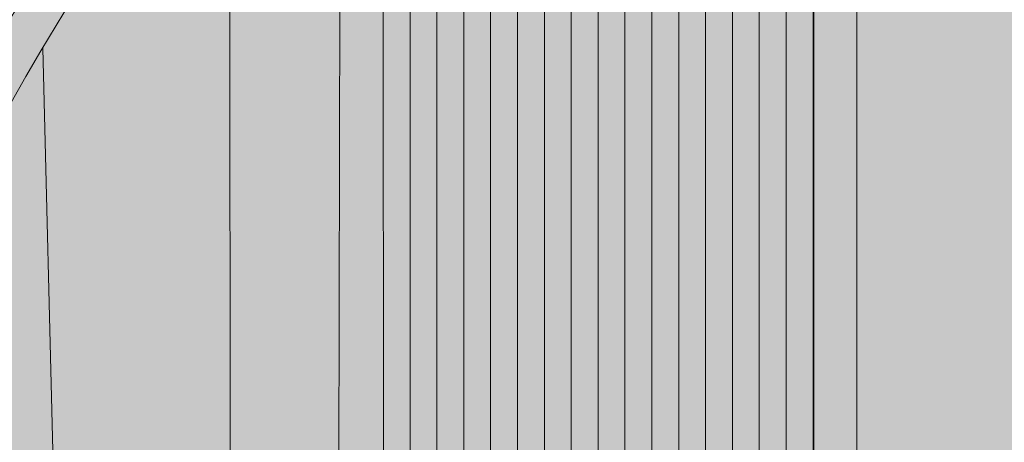
# Model space of a CAD drawing. Units: millimetres. Extents: x 11032 to 26788, y 3406 to 24505.
# Tile 9 of 78: x 15421 to 16566, y 8278 to 8770. Entities that reach past the tile are written whole.
import ezdxf

# ---------------------------------------------------------------- set-up
doc = ezdxf.new("R2010")
doc.units = ezdxf.units.MM
doc.header["$MEASUREMENT"] = 0
for name, color, linetype, lineweight in [('A-ANNO-DIMS', 2, 'Continuous', 18), ('A-GLAZ', 250, 'Continuous', 20), ('A-WALL-INTR', 8, 'Continuous', 18)]:
    doc.layers.add(name, color=color, linetype=linetype, lineweight=lineweight)
for name, color, linetype, lineweight, true_color in [('A-FNSH-INTR-PATT', 253, 'Continuous', 13, 0xc2b29b), ('A-GLAZ-FRAM-PATT', 250, 'Continuous', 13, 0x262627), ('A-WALL-INTR-PATT', 251, 'Continuous', 13, 0x6c6b6a)]:
    doc.layers.add(name, color=color, linetype=linetype, lineweight=lineweight, true_color=true_color)
doc.styles.get("Standard").update_dxf_attribs({"font": 'arial.ttf'})
doc.dimstyles.get("Standard").update_dxf_attribs({"dimtxt": 150, "dimasz": 100, "dimexe": 10, "dimexo": 5, "dimgap": 5, "dimtad": 0, "dimtih": 1, "dimtoh": 1, "dimdec": 0, "dimzin": 0, "dimdsep": 46, "dimtxsty": 'Standard', "dimcen": 0.09, "dimadec": 0, "dimazin": 0, "dimtfac": 1, "dimtdec": 0, "dimtofl": 0, "dimtmove": 0, "dimatfit": 3, "dimfxl": 1, "dimtolj": 1, "dimtzin": 0, "dimarcsym": 0})

# ---------------------------------------------------------------- blocks, each defined once
blk = doc.blocks.new('*D36')
at = {"layer": 'A-ANNO-DIMS', "color": 0, "lineweight": -2, "transparency": 16777216}
for p, q in [((12301.3, 17115.9), (12301.3, 24416.9)), ((25397.4, 4466.4), (25397.4, 24416.9)), ((12401.3, 24406.9), (18569.2, 24406.9)), ((25297.4, 24406.9), (19129.5, 24406.9))]:
    blk.add_line(p, q, dxfattribs=at)
at = {"layer": 'A-ANNO-DIMS', "color": 0, "transparency": 16777216}
for points in [[(12401.3, 24423.5), (12401.3, 24390.2), (12301.3, 24406.9)], [(25297.4, 24423.5), (25297.4, 24390.2), (25397.4, 24406.9)]]:
    blk.add_solid(points, dxfattribs=at)
at = {"layer": 'Defpoints', "color": 0, "transparency": 16777216}
for p in [(25397.4, 24406.9), (12301.3, 17110.9), (25397.4, 4461.4)]:
    blk.add_point(p, dxfattribs=at)
at = {"layer": 'A-ANNO-DIMS', "color": 0, "transparency": 16777216, "insert": (18849.3, 24406.9), "char_height": 150, "attachment_point": 5}
blk.add_mtext('\\A1;13096', dxfattribs=at)
blk = doc.blocks.new('*D37')
at = {"layer": 'A-ANNO-DIMS', "color": 0, "lineweight": -2, "transparency": 16777216}
for p, q in [((18087.7, 23450.4), (11334.8, 23450.4)), ((11344.8, 23350.4), (11344.8, 14037.5)), ((11344.8, 4561.4), (11344.8, 13874.3)), ((12927.7, 4461.4), (11334.8, 4461.4))]:
    blk.add_line(p, q, dxfattribs=at)
at = {"layer": 'A-ANNO-DIMS', "color": 0, "transparency": 16777216}
for points in [[(11328.1, 23350.4), (11361.4, 23350.4), (11344.8, 23450.4)], [(11328.1, 4561.4), (11361.4, 4561.4), (11344.8, 4461.4)]]:
    blk.add_solid(points, dxfattribs=at)
at = {"layer": 'Defpoints', "color": 0, "transparency": 16777216}
for p in [(11344.8, 23450.4), (18092.7, 23450.4), (12932.7, 4461.4)]:
    blk.add_point(p, dxfattribs=at)
at = {"layer": 'A-ANNO-DIMS', "color": 0, "transparency": 16777216, "insert": (11344.8, 13955.9), "char_height": 150, "attachment_point": 5}
blk.add_mtext('\\A1;18989', dxfattribs=at)
blk = doc.blocks.new('*D49')
at = {"layer": 'A-ANNO-DIMS', "color": 0, "lineweight": -2, "transparency": 16777216}
for p, q in [((17953.5, 10206.4), (17953.5, 3494.9)), ((14996.4, 6406.4), (14996.4, 3494.9)), ((15096.4, 3504.9), (16244.7, 3504.9)), ((17853.5, 3504.9), (16705.2, 3504.9))]:
    blk.add_line(p, q, dxfattribs=at)
at = {"layer": 'A-ANNO-DIMS', "color": 0, "transparency": 16777216}
for points in [[(15096.4, 3521.6), (15096.4, 3488.2), (14996.4, 3504.9)], [(17853.5, 3521.6), (17853.5, 3488.2), (17953.5, 3504.9)]]:
    blk.add_solid(points, dxfattribs=at)
at = {"layer": 'Defpoints', "color": 0, "transparency": 16777216}
for p in [(17953.5, 10211.4), (14996.4, 6411.4), (17953.5, 3504.9)]:
    blk.add_point(p, dxfattribs=at)
at = {"layer": 'A-ANNO-DIMS', "color": 0, "transparency": 16777216, "insert": (16474.9, 3504.9), "char_height": 150, "attachment_point": 5}
blk.add_mtext('\\A1;2957', dxfattribs=at)
blk = doc.blocks.new('*D57')
at = {"layer": 'A-ANNO-DIMS', "color": 0, "lineweight": -2, "transparency": 16777216}
for p, q in [((14994.7, 7266.4), (14994.7, 24416.9)), ((20894.7, 7266.4), (20894.7, 24416.9)), ((15094.7, 24406.9), (17716, 24406.9)), ((20794.7, 24406.9), (18173.4, 24406.9))]:
    blk.add_line(p, q, dxfattribs=at)
at = {"layer": 'A-ANNO-DIMS', "color": 0, "transparency": 16777216}
for points in [[(15094.7, 24423.5), (15094.7, 24390.2), (14994.7, 24406.9)], [(20794.7, 24423.5), (20794.7, 24390.2), (20894.7, 24406.9)]]:
    blk.add_solid(points, dxfattribs=at)
at = {"layer": 'Defpoints', "color": 0, "transparency": 16777216}
for p in [(20894.7, 24406.9), (14994.7, 7261.4), (20894.7, 7261.4)]:
    blk.add_point(p, dxfattribs=at)
at = {"layer": 'A-ANNO-DIMS', "color": 0, "transparency": 16777216, "insert": (17944.7, 24406.9), "char_height": 150, "attachment_point": 5}
blk.add_mtext('\\A1;5900', dxfattribs=at)
blk = doc.blocks.new('*D60')
at = {"layer": 'A-ANNO-DIMS', "color": 0, "lineweight": -2, "transparency": 16777216}
for p, q in [((14994.7, 7266.4), (14994.7, 24416.9)), ((16344.7, 7266.4), (16344.7, 24416.9)), ((15094.7, 24406.9), (15448, 24406.9)), ((16244.7, 24406.9), (15891.4, 24406.9))]:
    blk.add_line(p, q, dxfattribs=at)
at = {"layer": 'A-ANNO-DIMS', "color": 0, "transparency": 16777216}
for points in [[(15094.7, 24423.5), (15094.7, 24390.2), (14994.7, 24406.9)], [(16244.7, 24423.5), (16244.7, 24390.2), (16344.7, 24406.9)]]:
    blk.add_solid(points, dxfattribs=at)
at = {"layer": 'Defpoints', "color": 0, "transparency": 16777216}
for p in [(16344.7, 24406.9), (14994.7, 7261.4), (16344.7, 7261.4)]:
    blk.add_point(p, dxfattribs=at)
at = {"layer": 'A-ANNO-DIMS', "color": 0, "transparency": 16777216, "insert": (15669.7, 24406.9), "char_height": 150, "attachment_point": 5}
blk.add_mtext('\\A1;1350', dxfattribs=at)
blk = doc.blocks.new('*D69')
at = {"layer": 'A-ANNO-DIMS', "color": 0, "lineweight": -2, "transparency": 16777216}
for p, q in [((13957, 9938), (14057, 9938)), ((14057, 9938), (15432.5, 8991)), ((17944.6, 7261.4), (17944.8, 7261.4)), ((17944.7, 7261.3), (17944.7, 7261.5))]:
    blk.add_line(p, q, dxfattribs=at)
at = {"layer": 'A-ANNO-DIMS', "color": 0, "transparency": 16777216}
blk.add_solid([(15442, 9004.7), (15423.1, 8977.2), (15514.9, 8934.2)], dxfattribs=at)
at = {"layer": 'Defpoints', "color": 0, "transparency": 16777216}
for p in [(15514.9, 8934.2), (17944.7, 7261.4)]:
    blk.add_point(p, dxfattribs=at)
at = {"layer": 'A-ANNO-DIMS', "color": 0, "transparency": 16777216, "insert": (13494, 9938), "char_height": 150, "attachment_point": 5}
blk.add_mtext('\\A1;2X R2950', dxfattribs=at)

msp = doc.modelspace()

# ---------------------------------------------------------------- hatches: boundary and pattern name
at = {"layer": 'A-FNSH-INTR-PATT'}
h = msp.add_hatch(dxfattribs=at)
h.set_pattern_fill('ANSI31', color=256, scale=250, angle=45, style=0)
h.paths.add_polyline_path([(16344.704, 9680.076, 0.05653563), (15843.607, 9260.247), (15844.323, 7974.176), (15846.037, 7974.134), (15870.762, 8002.329), (15935.434, 8000.923, -0.11959168), (15991.005, 7804.617), (16002.667, 7804.617), (16022.264, 7889.032), (15962.718, 8099.323), (16012.167, 8155.712), (16076.839, 8154.307, -0.15483335), (16130.535, 7898.229, -0.14766935), (16201.035, 7901.954), (16191.395, 7843.208), (16202.533, 7804.617), (16299.12, 7804.617), (16297.929, 7808.825), (16344.704, 7862.164)])
at = {"layer": 'A-GLAZ-FRAM-PATT'}
h = msp.add_hatch(color=256, dxfattribs=at)
h.paths.add_polyline_path([(17944.704, 7311.399), (16344.704, 7311.399), (16344.704, 7261.399), (17944.704, 7261.399)], flags=17)
h.paths.add_polyline_path([(16344.704, 7311.399), (15045.135, 7311.399, -0.98290472), (20844.273, 7311.399), (19544.704, 7311.399), (19544.704, 7261.399), (20894.704, 7261.399, 0.51484406), (16985.951, 10051.255, 0.32026791), (14994.704, 7261.399), (16344.704, 7261.399)])
h.paths.add_polyline_path([(18744.704, 7311.399), (17944.704, 7311.399), (17944.704, 7261.399), (18744.704, 7261.399)], flags=17)
h.paths.add_polyline_path([(19544.704, 7311.399), (18744.704, 7311.399), (18744.704, 7261.399), (19544.704, 7261.399)], flags=17)
h.paths.add_polyline_path([(18694.704, 7361.399), (17994.704, 7361.399), (17994.704, 7311.399), (18694.704, 7311.399)], flags=17)
h.paths.add_polyline_path([(18744.704, 7361.399), (18694.704, 7361.399), (18694.704, 7311.399), (18744.704, 7311.399)], flags=17)
h.paths.add_polyline_path([(17194.704, 7361.399), (17144.704, 7361.399), (17144.704, 7311.399), (17194.704, 7311.399)], flags=17)
h.paths.add_polyline_path([(17431.432, 7361.399), (17194.704, 7361.399), (17194.704, 7311.399), (17431.699, 7311.399)], flags=17)
h.paths.add_polyline_path([(17894.704, 7361.399), (17431.432, 7361.399), (17431.699, 7311.399), (17894.704, 7311.399)], flags=17)
h.paths.add_polyline_path([(17944.704, 7361.399), (17894.704, 7361.399), (17894.704, 7311.399), (17944.704, 7311.399)], flags=17)
h.paths.add_polyline_path([(17994.704, 7361.399), (17944.704, 7361.399), (17944.704, 7311.399), (17994.704, 7311.399)], flags=17)
h = msp.add_hatch(color=256, dxfattribs=at)
h.paths.add_polyline_path([(16394.704, 9712.419, 0.00513365), (16344.704, 9680.076), (16344.704, 7862.164), (16347.378, 7865.214), (16394.704, 7864.185)])
h.paths.add_polyline_path([(17144.704, 10048.871, 0.02352245), (16886.403, 9961.399), (17094.704, 9961.399), (17094.704, 8264.696), (17144.704, 8264.696)])
h.paths.add_polyline_path([(18794.704, 9961.399), (19003.004, 9961.399, 0.02352245), (18744.704, 10048.871), (18744.704, 8264.696), (18794.704, 8264.696)])
h.paths.add_polyline_path([(19544.704, 9680.076, 0.00513365), (19494.704, 9712.419), (19494.704, 7793.43), (19544.704, 7793.43)])
h = msp.add_hatch(color=256, dxfattribs=at)
h.paths.add_polyline_path([(16734.609, 9896.863, 0.03337538), (16394.704, 9712.419), (16394.704, 7804.617), (16431.407, 7804.617), (16458.237, 7920.19), (16398.691, 8130.481), (16448.141, 8186.871), (16512.813, 8185.465, -0.15483335), (16566.508, 7929.387, -0.14766935), (16637.008, 7933.112), (16627.369, 7874.366), (16647.499, 7804.617), (16742.939, 7804.617)])
h.paths.add_polyline_path([(17094.704, 9961.399), (16886.403, 9961.399, 0.01422214), (16734.609, 9896.863), (16741.107, 8264.696), (17094.704, 8264.696)])
h.paths.add_polyline_path([(17417.202, 10027.292), (17194.704, 10011.399), (17194.704, 8264.696), (17426.61, 8264.696)])
h.paths.add_polyline_path([(17144.704, 8239.696), (17094.704, 8239.696), (17094.704, 7361.399), (16394.704, 7361.399), (16394.704, 7493.572), (16379.987, 7430.181), (16369.733, 7430.232), (16394.704, 7537.793), (16394.704, 7559.524), (16359.112, 7561.363), (16344.704, 7499.3), (16344.704, 7311.399), (17144.704, 7311.399)])
h.paths.add_polyline_path([(17194.704, 8239.696), (17144.704, 8239.696), (17144.704, 7361.399), (17194.704, 7361.399)])
at = {"layer": 'A-WALL-INTR-PATT'}
for points in [[(16344.704, 9680.076, 0.05653563), (15843.607, 9260.247), (15844.323, 7974.176), (15846.037, 7974.134), (15870.762, 8002.329), (15935.434, 8000.923, -0.11959168), (15991.005, 7804.617), (16002.667, 7804.617), (16022.264, 7889.032), (15962.718, 8099.323), (16012.167, 8155.712), (16076.839, 8154.307, -0.15483335), (16130.535, 7898.229, -0.14766935), (16201.035, 7901.954), (16191.395, 7843.208), (16202.533, 7804.617), (16299.12, 7804.617), (16297.929, 7808.825), (16344.704, 7862.164)], [(15843.607, 9260.247, 0.0062633), (15794.195, 9206.987), (15790.874, 7662.689, -0.11121794), (15844.495, 7664.925), (15844.384, 7864.461), (15821.312, 7945.94), (15844.324, 7972.181)], [(15794.195, 9206.987, 0.0171928), (15665.595, 9054.627), (15665.763, 7917.077), (15727.534, 7915.735, -0.15483335), (15781.23, 7659.657, -0.02070391), (15790.874, 7662.689)], [(15665.595, 9054.627, 0.03326569), (15447.906, 8736.527), (15472.44, 7764.657), (15521.889, 7821.046), (15586.562, 7819.64, -0.15483335), (15640.257, 7563.563, -0.02875494), (15653.713, 7567.556), (15665.807, 7619.654), (15665.799, 7675.745), (15613.413, 7860.751), (15662.862, 7917.14), (15665.763, 7917.077)], [(15447.906, 8736.527, 0.02717166), (15302.659, 8457.059), (15381.661, 7740.545), (15467.334, 7311.399), (15790.119, 7311.399), (15790.667, 7566.433), (15778.696, 7607.911), (15725.317, 7610.669), (15701.389, 7507.6), (15736.743, 7385.107), (15726.32, 7385.159), (15696.749, 7487.614), (15695.471, 7482.107), (15685.217, 7482.158), (15691.06, 7507.327), (15690.552, 7509.088), (15650.881, 7511.137), (15649.743, 7506.234), (15684.627, 7385.366), (15674.204, 7385.418), (15645.103, 7486.248), (15644.2, 7482.362), (15633.946, 7482.413), (15639.413, 7505.961), (15637.723, 7511.817), (15584.344, 7514.575), (15554.498, 7386.013), (15544.244, 7386.064), (15574.2, 7515.099), (15533.623, 7517.195), (15503.228, 7386.268), (15492.974, 7386.319), (15531.986, 7554.365), (15472.44, 7764.657)]]:
    msp.add_hatch(color=256, dxfattribs=at).paths.add_polyline_path(points)

# ---------------------------------------------------------------- linework, layer by layer
at = {"layer": 'A-GLAZ'}
for p, q in [((16394.704, 7361.399), (16394.704, 9712.419)), ((16344.704, 7261.399), (16344.704, 9680.076))]:
    msp.add_line(p, q, dxfattribs=at)
for radius, start, end in [(2900, 0.987907, 179.012093), (2950, 108.965621, 181.942602)]:
    msp.add_arc((17944.704, 7261.399), radius, start, end, dxfattribs=at)
at = {"layer": 'A-WALL-INTR'}
for p, q in [((15843.607, 9260.247), (15844.691, 7311.399)), ((15790.119, 7311.399), (15794.195, 9206.987)), ((15665.595, 9054.627), (15665.815, 7569.766)), ((15447.906, 8736.527), (15472.44, 7764.657))]:
    msp.add_line(p, q, dxfattribs=at)

# ---------------------------------------------------------------- dimensions: what is measured, and where the dimension line sits
at = {"layer": 'A-ANNO-DIMS'}
for base, p1, p2, picture, middle in [((25397.404, 24406.858), (12301.265, 17110.885), (25397.404, 4461.399), '*D36', (18849.334, 24406.858)), ((20894.704, 24406.858), (14994.704, 7261.399), (20894.704, 7261.399), '*D57', (17944.704, 24406.858)), ((16344.704, 24406.858), (14994.704, 7261.399), (16344.704, 7261.399), '*D60', (15669.704, 24406.858)), ((17953.455, 3504.899), (14996.399, 6411.399), (17953.455, 10211.41), '*D49', (16474.927, 3504.899))]:
    dim = msp.add_linear_dim(base=base, p1=p1, p2=p2, dimstyle='Standard', override={"dimdec": 0, "dimlfac": 1, "dimrnd": 0, "dimzin": 0, "dimdsep": 46, "dimlunit": 2}, dxfattribs=at)
    dim.commit()
    dim.dimension.update_dxf_attribs({"geometry": picture, "text_midpoint": middle})
dim = msp.add_linear_dim(base=(11344.765, 23450.358), p1=(12932.665, 4461.399), p2=(18092.739, 23450.358), angle=90, dimstyle='Standard', override={"dimdec": 0, "dimlfac": 1, "dimrnd": 0, "dimzin": 0, "dimdsep": 46, "dimlunit": 2}, dxfattribs=at)
dim.commit()
dim.dimension.update_dxf_attribs({"geometry": '*D37', "text_midpoint": (11344.765, 13955.879)})
dim = msp.add_radius_dim(center=(17944.704, 7261.399), mpoint=(15514.87, 8934.244), text='2X <>', dimstyle='Standard', override={"dimdec": 0, "dimlfac": 1, "dimrnd": 0, "dimzin": 0, "dimdsep": 46, "dimlunit": 2}, dxfattribs=at)
dim.commit()
dim.dimension.update_dxf_attribs({"geometry": '*D69', "text_midpoint": (13494.04, 9937.951), "dimtype": 164})

doc.saveas('drawing.dxf')
